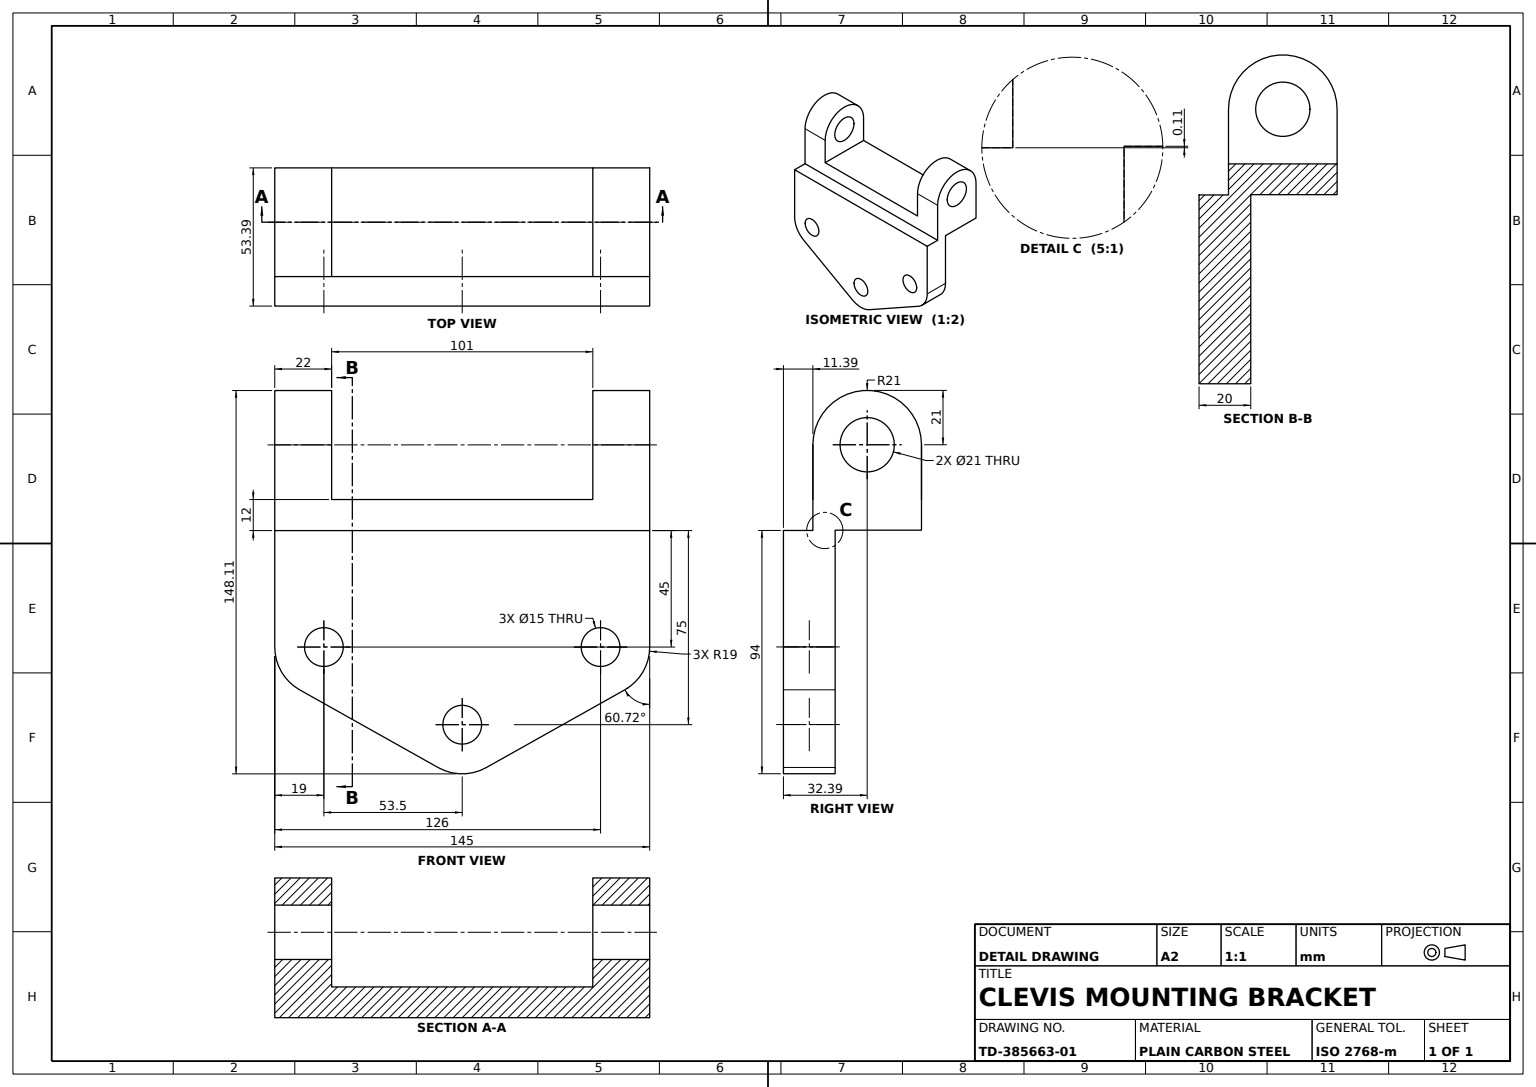
from build123d import *
from build123d.topology import SkipClean

# Parameters (mm, degrees)
BRACKET_PROFILE_SKETCH_R       = 10.5
BRACKET_BODY_145MM_DEPTH       = 72.5
PLATE_AND_LUG_OUTLINE_SKETCH_R = 7.5
PLATE_AND_LUG_OUTLINE_SKETCH_W = 101
PLATE_AND_LUG_OUTLINE_SKETCH_H = 63.401381975
OUTLINE_AND_HOLES_CUT_DEPTH    = 145
LUG_REGION_BOSS_DEPTH          = 20


with BuildPart() as part:
    # Bracket Profile Sketch → Bracket Body 145mm (new, symmetric)
    with BuildSketch(Plane(origin=(0, 0, 0), x_dir=(0, 0, -1), z_dir=(1, 0, 0))):
        with BuildLine():
            Line((-8.607818135, 33), (-8.607818135, -0.114515686))
            Line((-8.607818135, -0.114515686), (-20, -0.114515686))
            Line((-20, -0.114515686), (-20, -75.114515686))
            Line((-20, -75.114515686), (0, -75.114515686))
            Line((0, -75.114515686), (0, 0))
            Line((0, 0), (33.392181865, 0))
            Line((33.392181865, 0), (33.392181865, 33))
            ThreePointArc((33.392181865, 33), (12.392181865, 54), (-8.607818135, 33))
        make_face()
        with Locations((12.392181865, 33)):
            Circle(BRACKET_PROFILE_SKETCH_R, mode=Mode.SUBTRACT)
    extrude(amount=BRACKET_BODY_145MM_DEPTH, both=True)

    # Plate and Lug Outline Sketch → Outline and Holes Cut (cut)
    with BuildSketch(Plane.XY.offset(20)):
        with BuildLine():
            Line((-38.846882472, -75.114515686), (-62.792895003, -61.686845107))
            ThreePointArc((-62.792895003, -61.686845107), (-69.894587599, -54.717509879), (-72.5, -45.114515686))
            Line((-72.5, -45.114515686), (-72.5, -75.114515686))
            Line((-72.5, -75.114515686), (-38.846882472, -75.114515686))
        make_face()
        with BuildLine():
            Line((62.792895003, -61.686845107), (38.846882472, -75.114515686))
            Line((38.846882472, -75.114515686), (72.5, -75.114515686))
            Line((72.5, -75.114515686), (72.5, -45.114515686))
            ThreePointArc((72.5, -45.114515686), (69.894587599, -54.717509879), (62.792895003, -61.686845107))
        make_face()
        with Locations((53.5, -45.114515686)):
            Circle(PLATE_AND_LUG_OUTLINE_SKETCH_R)
        with BuildLine():
            ThreePointArc((0, -67.614515686), (-5.303300859, -69.811214827), (-7.5, -75.114515686))
            Line((-7.5, -75.114515686), (0, -75.114515686))
            Line((0, -75.114515686), (0, -67.614515686))
        make_face()
        with BuildLine():
            ThreePointArc((7.5, -75.114515686), (5.303300859, -69.811214827), (0, -67.614515686))
            Line((0, -67.614515686), (0, -75.114515686))
            Line((0, -75.114515686), (7.5, -75.114515686))
        make_face()
        with BuildLine():
            Line((0, -75.114515686), (-7.5, -75.114515686))
            ThreePointArc((-7.5, -75.114515686), (0, -82.614515686), (7.5, -75.114515686))
            Line((7.5, -75.114515686), (0, -75.114515686))
        make_face()
        with Locations((-53.5, -45.114515686)):
            Circle(PLATE_AND_LUG_OUTLINE_SKETCH_R)
        with Locations((0, 43.586175301)):
            Rectangle(PLATE_AND_LUG_OUTLINE_SKETCH_W, PLATE_AND_LUG_OUTLINE_SKETCH_H)
    extrude(amount=-OUTLINE_AND_HOLES_CUT_DEPTH, mode=Mode.SUBTRACT)

    # Sketch2_3 → Lug Region Boss (add)
    with SkipClean():  # the faces are left unmerged after this step: merging them gives an invalid solid
        with BuildSketch(Plane.XY.offset(20)):
            with BuildLine():
                Line((-7.5, -75.114515686), (-38.846882472, -75.114515686))
                Line((-38.846882472, -75.114515686), (-9.292895003, -91.686845107))
                ThreePointArc((-9.292895003, -91.686845107), (0, -94.114515686), (9.292895003, -91.686845107))
                Line((9.292895003, -91.686845107), (38.846882472, -75.114515686))
                Line((38.846882472, -75.114515686), (7.5, -75.114515686))
                ThreePointArc((7.5, -75.114515686), (0, -82.614515686), (-7.5, -75.114515686))
            make_face()
        extrude(amount=-LUG_REGION_BOSS_DEPTH)


solid = part.part
